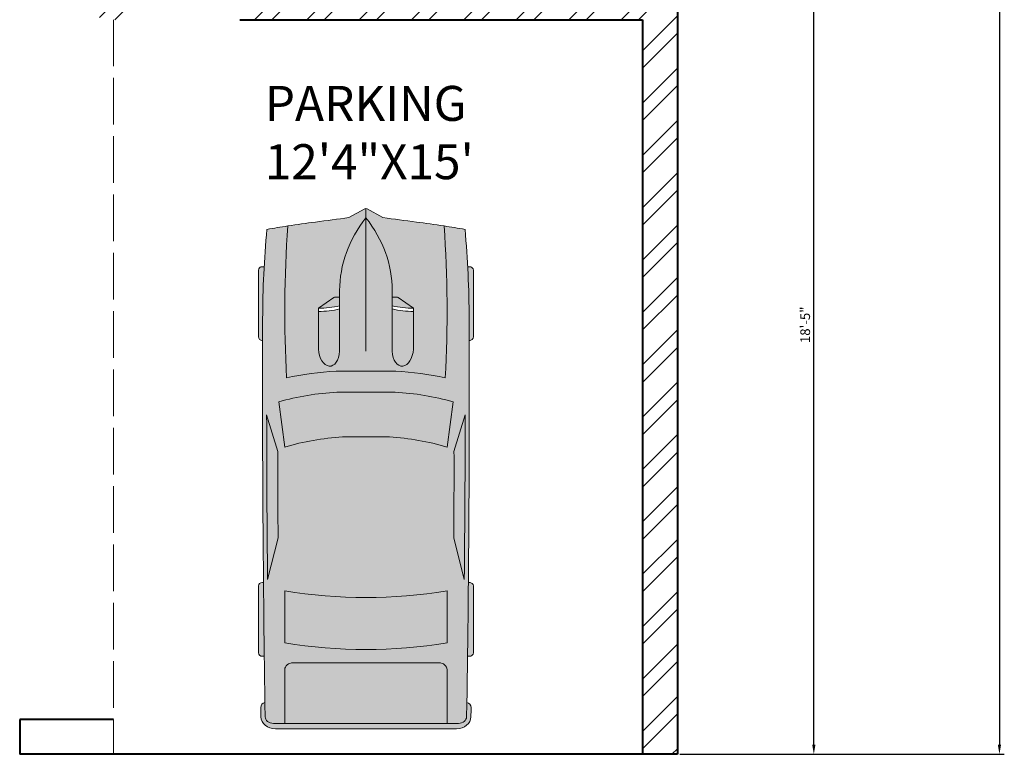
# Model space of a CAD drawing. Units: inches. Extents: x 1143 to 1626, y 7431 to 8140.
# Tile 2 of 4: x 1373 to 1626, y 7467 to 7656. Entities that reach past the tile are written whole.
import ezdxf

# ---------------------------------------------------------------- set-up
doc = ezdxf.new("R2010")
doc.units = ezdxf.units.IN
doc.linetypes.add('ACAD_ISO02W100', pattern=[15, 12, -3])
for name, color, linetype, lineweight in [('A-ANNO-DIMS', 4, 'Continuous', 18), ('A-EQPM-PATT', 9, 'Continuous', 13), ('A-EQPM-VEHC', 8, 'Continuous', 18), ('A-FLOR-PRKG', 2, 'ACAD_ISO02W100', 18), ('A-WALL', 2, 'Continuous', 40), ('A-WALL-PATT', 7, 'Continuous', 13)]:
    doc.layers.add(name, color=color, linetype=linetype, lineweight=lineweight)
doc.layers.add('A-AREA-IDEN', color=40, linetype='Continuous', lineweight=25, true_color=0xf8d731)
doc.styles.get("Standard").update_dxf_attribs({"font": 'arial.ttf'})
doc.dimstyles.new('ISO-25', dxfattribs={"dimtxt": 2.5, "dimasz": 2.5, "dimexe": 1.25, "dimexo": 0.625, "dimtad": 1, "dimdec": 0, "dimlunit": 3, "dimtxsty": 'Standard', "dimcen": 2.5, "dimadec": 0, "dimazin": 0, "dimtfac": 1, "dimtdec": 0, "dimtmove": 0, "dimatfit": 3, "dimfxl": 1, "dimarcsym": 0})

# ---------------------------------------------------------------- blocks, each defined once
blk = doc.blocks.new('*U56')
for p, q in [((536.0433148737552, 950.1792138851854), (536.0433148737552, 935.5404748014407)), ((1182.463644577746, 987.7673041878503), (567.7039087844591, 987.7673041878503)), ((1214.124238488447, 949.7089586534819), (1214.124238488447, 950.1792138851854)), ((2234.827175480885, 809.5287016048088), (1898.878785383111, 912.4126225124705)), ((3440.463608272525, 941.6679440245914), (3440.463608272525, 950.1792138851854)), ((3472.124202183229, 987.7673041878503), (4086.88393797651, 987.767304187848)), ((4118.544531887212, 950.1792138851804), (4118.544531887212, 934.0601128753084)), ((3411.559256322833, 904.3494681924599), (3029.921878250559, 807.1504809911063)), ((4736.411271353851, -850.8646766016326), (4736.411271353883, 850.864676601626)), ((4785.334832293326, -832.0706314503777), (4785.334832293357, 832.0706314502926)), ((1778.76917512805, 801.0177247054045), (2194.716249451875, 745.5217224176465)), ((3515.941238262737, 745.5217224176508), (3994.062813016633, 745.5217224176508)), ((4736.411271353883, 745.5217224176529), (4242.012185201922, 745.5217224176529)), ((4178.690997380514, 670.345541812321), (4178.690997380509, -670.3455418123318)), ((819.5542361210883, 295.2827619512633), (917.6699264680983, 436.1082195367583)), ((917.6699264680983, 436.1082195367583), (1293.848362214069, 436.1082195367583)), ((815.9220749762081, 241.4481679439487), (815.9220749762081, 283.3039660446585)), ((1496.485716216861, -273.6820371142997), (1496.485716216861, 273.6820371142868)), ((756.2288711996046, 241.4481679439487), (1312.764151599097, 241.4481679439487)), ((1690.372337881975, -267.4332505757059), (1690.372337881975, 267.4332505756928)), ((2101.521373270556, 215.7994139342878), (2101.521373270556, -215.7994139342835)), ((4736.411271353883, -267.4332505757059), (4736.411271353883, 267.4332505756928)), ((82.96813941916749, 155.6585683733955), (2.596917328392246, 10.3141998552517)), ((-1.1252e-12, -6.4972e-12), (1312.764151599097, -6.4972e-12)), ((2.596917328392246, -10.31419985525964), (82.96813941916749, -155.6585683734063)), ((756.2288711996046, -241.4481679439617), (1312.764151599097, -241.4481679439617)), ((815.9220749762081, -241.4481679439617), (815.9220749762081, -283.3039660446715)), ((819.5542361210883, -295.2827619512763), (917.6699264680983, -436.1082195367712)), ((917.6699264680983, -436.1082195367712), (1293.848362214069, -436.1082195367712)), ((2194.716249451869, -745.5217224176688), (1778.769175128041, -801.0177247054262)), ((2234.827175480882, -809.5287016048153), (1898.878785383109, -912.4126225124726)), ((3411.559256322828, -904.349468192473), (3029.921878250557, -807.150480991115)), ((3994.062813016633, -745.5217224176616), (3515.941238262737, -745.5217224176638)), ((4242.012185201917, -745.5217224176638), (4736.411271353857, -745.5217224176594)), ((536.0433148737552, -950.1792138851984), (536.0433148737552, -935.5404748014537)), ((1182.463644577746, -987.7673041878633), (567.7039087844591, -987.7673041878633)), ((1214.124238488447, -949.7089586534948), (1214.124238488447, -950.1792138851984)), ((3440.463608272523, -941.6679440246044), (3440.463608272523, -950.1792138851984)), ((3472.124202183229, -987.7673041878633), (4086.883937976504, -987.767304187861)), ((4118.544531887212, -950.1792138851933), (4118.544531887212, -934.0601128753214))]:
    blk.add_line(p, q)
for centre, major_axis, ratio, start_param, end_param in [((6757.162543998887, -699.1204428451242), (4.9938223e-09, 7958.017136535005), 0.8423038695435286, 1.367075990158062, 1.391760499156098), ((1046.255263051279, -12467.92283887244), (3.2861e-12, 13417.14359589015), 0.8423038695439741, 0.0028100083536837, 0.0755983031096952), ((567.7039087844591, 950.1792138851861), (5.296e-13, -37.5880903026662), 0.842303869543976, 3.141592653589776, 4.712388980384677), ((1637.842620806017, -268112.68896731), (4.8454159e-09, 269062.8681811952), 0.842303869543847, -0.0133969486112073, 0.0027970409639888), ((1182.463644577746, 950.1792138851861), (5.601e-13, 37.58809030266621), 0.8423038695439758, -1.570796326794884, 1.73e-14), ((1637.842620802809, -268112.6889680619), (4.87113144e-08, -269025.2800916445), 0.8423038695482963, 3.133765086725325, 3.140440689641252), ((3472.124202183229, 950.1792138851861), (5.988e-12, -37.5880903026662), 0.8423038695439762, 3.141592653589603, 4.712388980384554), ((4086.88393797651, 950.179213885181), (1.4197e-12, 37.5880903026662), 0.842303869543976, -1.570796326794865, 4.44e-14), ((4587.952203166941, 910.2894362332722), (1.8792e-12, 56.38213545399769), 0.8423038695439691, -0.0130174256259048, 1.249894140392862), ((1637.84262086767, -268131.4830124673), (3.42859201765e-05, 269120.9512111412), 0.8423038681351471, -0.0133969484821159, -0.0130174254969711), ((4673.090083532475, 850.8646766015395), (7.5e-15, -75.17618060533067), 0.8423038695439952, 1.570796326796048, 3.128195704978389), ((4673.090083532448, 832.070631450172), (2.1733e-12, -133.2592106239272), 0.8423038695439737, 1.570796326795794, 3.128195704978164), ((951.8333444315502, -15086.63944974413), (1.5767e-12, -15832.53653317094), 0.8423038695439826, 3.09604606856106, 3.200911180495224), ((3413.769624379244, 136.8410185571329), (1.08602e-11, -2280.347340451234), 0.84230386954398, 4.44948196380473, 4.652344057257214), ((3436.395912346701, 136.8410185571553), (5.76965e-11, 2077.023647078763), 0.8423038695439563, 1.245306111696802, 1.507880129813836), ((3799.722190048092, 71.1058404433382), (2.17448e-11, -2021.323467232052), 0.842303869543983, 4.372215489277867, 4.640744122441986), ((2433.035484508693, -93125.37499596032), (4.952654e-09, -93935.19844392464), 0.8423038695446962, 3.134048706297306, 3.14409775411291), ((433.884764992104, -3.6096e-12), (1.7438e-12, 3734.255266801694), 0.8423038695439766, 4.511394369635731, 4.913383591133647), ((912.0063397460013, -3.6096e-12), (1.7438e-12, 3734.255266801694), 0.8423038695439766, 4.511394369635731, 4.913383591133647), ((4242.012185201922, 670.3455418123216), (3.5405e-12, 75.17618060533239), 0.842303869543976, 5.55e-14, 1.57079632679492), ((6583.045501169266, -699.1204428451198), (3.826807e-09, -7754.693443154298), 0.8423038695443791, 4.528606069860317, 4.561837674556238), ((-5194.164488957196, 1330.879982200552), (1.0466145e-09, -6374.389491984369), 0.8423038695441164, 1.385369446298923, 1.434372047871027), ((331.12799165183, 432.0470009052715), (3.125e-11, 696.3661584994836), 0.8423038695439277, 4.435146050259648, 4.718221029521873), ((360.7019022476185, 432.0470009052715), (3.125e-11, 696.3661584994836), 0.8423038695439277, 4.435146050259648, 4.718221029521873), ((1290.073045555822, 338.7781937403542), (161.0379696969085, -9.057857958340485), 0.6038335755719145, -1.39555193967809, 1.581314658479915), ((831.7523719315589, 283.3039660446593), (3.3347e-12, 18.79404515133458), 0.8423038695439091, 0.8797135699495516, 1.570796326795045), ((756.2288711996046, -1185.240851913765), (1.2998e-12, 1426.689019857713), 0.842303869543976, 7e-16, 0.5903187773915901), ((15.83029695535095, -3.6096e-12), (1.9e-15, -18.79404515133476), 0.842303869543842, 4.131459131953847, 5.293318828815531), ((756.2288711996046, 1185.240851913753), (1.01699e-11, 1426.689019857713), 0.8423038695439736, 2.55127387619821, 3.141592653589801), ((-5194.164488957196, -1330.879982200562), (1.0234792e-09, 6374.389491984348), 0.8423038695441192, -1.43437204787103, -1.385369446298926), ((331.12799165183, -432.0470009052816), (3.1922e-11, -696.3661584994801), 0.842303869543932, 1.564964277657711, 1.848039256919935), ((360.7019022476185, -432.0470009052816), (3.1922e-11, -696.3661584994801), 0.842303869543932, 1.564964277657711, 1.848039256919935), ((3436.395912346742, -136.8410185572101), (8.13766e-11, -2077.023647078826), 0.8423038695439492, -1.50788012981387, -1.245306111696839), ((3799.722190048497, -71.10584044329416), (1.038796e-10, -2021.323467232635), 0.8423038695439419, -1.499151468852248, -1.230622835688196), ((831.7523719315589, -283.3039660446737), (3.3028e-12, -18.79404515133458), 0.8423038695439093, 4.712388980384541, 5.403471737230034), ((3413.769624379237, -136.841018557156), (1.090899e-10, -2280.347340451348), 0.8423038695439354, -1.510751403667474, -1.307889310215002), ((6583.045501169163, 699.1204428449458), (2.756795e-10, 7754.693443157768), 0.8423038695439974, 1.721347632622872, 1.754579237318777), ((6757.162543998887, 699.1204428451076), (2.2231118e-09, 7958.017136528592), 0.8423038695441819, 1.749832154434603, 1.774516663432659), ((951.8333444315729, 15086.63944974408), (2.97009e-11, -15832.5365331709), 0.8423038695439528, -0.0593185269054384, 0.0455465850287298), ((4242.012185201917, -670.3455418123318), (2.579e-13, -75.17618060533128), 0.8423038695439885, 4.712388980384686, 6.283185307179581), ((2433.03548450906, 93125.37499596029), (4.1600574e-09, -93935.19844392457), 0.8423038695447548, -0.0025051005232382, 0.007543947292366), ((1637.842620803916, 268112.6889680615), (4.0766478e-08, -269025.280091644), 0.8423038695397146, 0.0011519639481523, 0.0078275668641468), ((4673.090083532448, -850.8646766015358), (2.354e-13, 75.17618060532999), 0.8423038695439732, 3.154989602201626, 4.71238898038339), ((4673.090083532349, -832.0706314501077), (6.1679e-12, -133.2592106240062), 0.8423038695439807, 0.0133969486110846, 1.570796326792831), ((1046.255263051284, 12467.92283887242), (3.49903e-10, -13417.14359589015), 0.8423038695440652, -0.0755983031097181, -0.0028100083537155), ((567.7039087844591, -950.1792138851977), (5.601e-13, 37.58809030266621), 0.8423038695439758, 1.570796326794908, 3.14159265358981), ((1637.842620801787, 268112.6889680619), (1.55395844e-08, 269062.868181947), 0.8423038695458147, 3.138795612625926, 3.154989602201039), ((1182.463644577746, -950.1792138851977), (5.296e-13, -37.5880903026662), 0.842303869543976, -1.69e-14, 1.570796326794884), ((3472.124202183229, -950.1792138851955), (3.96e-13, -37.58809030266733), 0.8423038695440105, -1.570796326794875, -1.27e-14), ((4086.883937976504, -950.1792138851933), (5.0003e-12, 37.58809030266732), 0.8423038695440109, 3.141592653589951, 4.712388980384771), ((4587.952203166856, -910.2894362333229), (5.777e-12, -56.38213545402103), 0.8423038695439803, -1.249894138785958, 0.0130174256254374), ((1637.842620726191, 268131.4830135791), (2.37878358395e-05, 269120.9512123862), 0.8423038705260315, 3.154610079306566, 3.154989602290631)]:
    blk.add_ellipse(centre, major_axis=major_axis, ratio=ratio, start_param=start_param, end_param=end_param)
at = {"extrusion": (0, 0, -1)}
blk.add_ellipse((1290.073045555822, -338.7781937403665), major_axis=(161.0379696969085, 9.057857958340424), ratio=0.6038335755719145, start_param=-1.39555193967809, end_param=1.581314658479915, dxfattribs=at)
blk = doc.blocks.new('*D59')
at = {"layer": 'A-ANNO-DIMS', "color": 0, "lineweight": -2, "transparency": 16777216}
for p, q in [((1542.475441917873, 8067.395884901202), (1625.931990479295, 8067.395884901202)), ((1624.681990479295, 8064.895884901202), (1624.681990479295, 7469.895884901203)), ((1542.475441917873, 7467.395884901204), (1625.931990479295, 7467.395884901204))]:
    blk.add_line(p, q, dxfattribs=at)
at = {"layer": 'A-ANNO-DIMS', "color": 0, "transparency": 16777216}
for points in [[(1624.265323812629, 8064.895884901202), (1625.098657145962, 8064.895884901202), (1624.681990479295, 8067.395884901202)], [(1624.265323812629, 7469.895884901203), (1625.098657145963, 7469.895884901203), (1624.681990479295, 7467.395884901204)]]:
    blk.add_solid(points, dxfattribs=at)
at = {"layer": 'Defpoints', "color": 0, "transparency": 16777216}
for p in [(1541.850441917873, 8067.395884901202), (1541.850441917873, 7467.395884901204), (1624.681990479295, 7467.395884901204)]:
    blk.add_point(p, dxfattribs=at)
at = {"layer": 'A-ANNO-DIMS', "color": 0, "transparency": 16777216, "insert": (1615.88782267575, 7767.395884901201), "char_height": 2.5, "attachment_point": 5, "rotation": 90}
blk.add_mtext("{\\H6.4x;50'}", dxfattribs=at)
blk = doc.blocks.new('*D94')
at = {"layer": 'A-ANNO-DIMS', "color": 0, "lineweight": -2, "transparency": 16777216}
for p, q in [((1542.475442000001, 7688.395885000004), (1578.200442000001, 7688.395885000004)), ((1576.950442000002, 7469.895885000004), (1576.950442000002, 7685.895885000004)), ((1542.475442000001, 7467.395885000003), (1578.200442000002, 7467.395885000003))]:
    blk.add_line(p, q, dxfattribs=at)
at = {"layer": 'A-ANNO-DIMS', "color": 0, "transparency": 16777216}
for points in [[(1576.533775333335, 7685.895885000004), (1577.367108666668, 7685.895885000004), (1576.950442000002, 7688.395885000004)], [(1576.533775333335, 7469.895885000004), (1577.367108666669, 7469.895885000004), (1576.950442000002, 7467.395885000003)]]:
    blk.add_solid(points, dxfattribs=at)
at = {"layer": 'Defpoints', "color": 0, "transparency": 16777216}
for p in [(1541.850442000001, 7688.395885000004), (1576.950442000002, 7688.395885000004), (1541.850442000001, 7467.395885000003)]:
    blk.add_point(p, dxfattribs=at)
at = {"layer": 'A-ANNO-DIMS', "color": 0, "transparency": 16777216, "insert": (1575.049009530699, 7577.895885000002), "char_height": 2.5, "attachment_point": 5, "rotation": 90}
blk.add_mtext('18\'-5"', dxfattribs=at)

msp = doc.modelspace()

# ---------------------------------------------------------------- hatches: boundary and pattern name
at = {"layer": 'A-EQPM-PATT'}
h = msp.add_hatch(color=256, dxfattribs=at)
h.dxf.hatch_style = 1
edge = h.paths.add_edge_path()
edge.add_ellipse((1039.678384205543, 7581.215646983221), major_axis=(442.95140415634, 3.6663e-12), ratio=0.8423038695438162, start_angle=-2.198540565955638, end_angle=2.863714607837108)
edge.add_ellipse((1442.202119620892, 7423.669613427368), major_axis=(216.9552770171625, 6.603309e-10), ratio=0.8423038695464521, start_angle=77.55537270638033, end_angle=79.79046100268101)
edge.add_ellipse((1498.996022280016, 7753.163986690991), major_axis=(178.3381184811209, 2.862326e-10), ratio=0.842303869545449, start_angle=257.4450673557707, end_angle=260.7434339927064, ccw=False)
edge.add_line((1466.116516563501, 7605.524137399554), (1462.050175583554, 7607.772706073581))
edge.add_ellipse((1461.761612263391, 7607.402472025788), major_axis=(-0.5258063780318869, 7.886e-13), ratio=0.8423038695429472, start_angle=232.0668695402551, end_angle=270.0000000000859)
edge.add_line((1461.761612263391, 7607.845360772635), (1461.761612263391, 7605.40214945713))
edge.add_ellipse((1428.601789861041, 7586.688129291778), major_axis=(-39.91488687339462, 4.1769e-12), ratio=0.8423038695440169, start_angle=180.000000000006, end_angle=209.4385695979854, ccw=False)
edge.add_line((1468.516676734435, 7586.688129291778), (1468.516676734435, 7585.01807545195))
edge.add_line((1468.516676734435, 7585.01807545195), (1469.811288061556, 7585.01807545195))
edge.add_ellipse((1469.687688372524, 7584.575186705103), major_axis=(0.5258063780289138, 6.2901e-12), ratio=0.8423038695477099, start_angle=45.519789116729726, end_angle=89.99999999931458, ccw=False)
edge.add_line((1470.022822572645, 7584.916457440465), (1473.962736688602, 7582.171446701479))
edge.add_line((1473.962736688602, 7582.171446701479), (1473.962736688602, 7571.646994982835))
edge.add_ellipse((1471.239706711519, 7571.752618097072), major_axis=(0.2534142834889348, 4.505405349943914), ratio=0.6038335755718542, start_angle=106.3425919543661, end_angle=270.9979857250239, ccw=False)
edge.add_line((1468.516676734435, 7571.117782531546), (1468.516676734435, 7586.688129291778))
edge.add_ellipse((1428.601789861041, 7586.688129291778), major_axis=(-39.91488687339462, 4.1769e-12), ratio=0.8423038695440169, start_angle=180.000000000006, end_angle=209.4385695979854)
edge.add_ellipse((1494.92143466574, 7586.688129291778), major_axis=(-39.9148868733946, 1.8282e-12), ratio=0.8423038695439518, start_angle=-29.43856959797676, end_angle=2.6254e-12)
edge.add_line((1455.006547792345, 7586.688129291778), (1455.006547792345, 7571.117782531546))
edge.add_ellipse((1452.283517815262, 7571.752618097072), major_axis=(-0.2534142834889348, 4.505405349943914), ratio=0.6038335755718542, start_angle=89.0020142749762, end_angle=253.6574080456339, ccw=False)
edge.add_line((1449.560487838178, 7571.646994982835), (1449.560487838178, 7582.171446701479))
edge.add_line((1449.560487838178, 7582.171446701479), (1453.595642479137, 7584.982813268593))
edge.add_ellipse((1453.835536154257, 7584.575186705103), major_axis=(-0.525806378028914, 6.2893e-12), ratio=0.8423038695477096, start_angle=-89.99999999931458, end_angle=-45.519789116729726, ccw=False)
edge.add_line((1453.835536154257, 7585.01807545195), (1455.006547792345, 7585.01807545195))
edge.add_line((1455.006547792345, 7585.01807545195), (1455.006547792345, 7586.688129291778))
edge.add_ellipse((1494.92143466574, 7586.688129291778), major_axis=(-39.9148868733946, 1.8282e-12), ratio=0.8423038695439518, start_angle=-29.438569597976823, end_angle=2.6716406864579767e-12, ccw=False)
edge.add_line((1461.761612263391, 7605.40214945713), (1461.761612263391, 7607.845360772635))
edge.add_ellipse((1461.761612263391, 7607.402472025788), major_axis=(-0.5258063780318869, 7.886e-13), ratio=0.8423038695429472, start_angle=270.0000000000859, end_angle=307.9331304599605)
edge.add_line((1461.473048943226, 7607.772706073581), (1457.406707963279, 7605.524137399554))
edge.add_ellipse((1424.527202246764, 7753.163986690991), major_axis=(-178.3381184811248, 2.85599e-10), ratio=0.8423038695454304, start_angle=99.25656600729332, end_angle=102.5549326442291, ccw=False)
edge.add_ellipse((1481.321104905884, 7423.669613427371), major_axis=(-216.9552770172325, 5.765085e-10), ratio=0.8423038695461753, start_angle=-79.79046100270455, end_angle=-77.55537270640374)
edge.add_ellipse((1883.844840321237, 7581.215646983221), major_axis=(-442.9514041563389, 7.3054e-12), ratio=0.8423038695438002, start_angle=-2.863714607836754, end_angle=2.198540565956014)
edge.add_ellipse((1457.933171938046, 7512.337351337953), major_axis=(-63.79792993373228, 4.06461e-11), ratio=0.8423038695444189, start_angle=-85.9175893088132, end_angle=-72.2800467772135, ccw=False)
edge.add_line((1454.104731612702, 7565.977751756898), (1469.418492914078, 7565.977751756898))
edge.add_ellipse((1465.590052588734, 7512.337351337953), major_axis=(63.79792993373165, 4.44426e-11), ratio=0.8423038695444265, start_angle=72.2800467772093, end_angle=85.91758930880928, ccw=False)
edge = h.paths.add_edge_path()
edge.add_ellipse((1480.516061267415, 7489.165372259944), major_axis=(-2.103225512126755, 1.679e-12), ratio=0.842303869543697, start_angle=180.0000000000457, end_angle=270.0000000000457)
edge.add_line((1480.516061267415, 7490.936927247331), (1443.007163259365, 7490.936927247331))
edge.add_ellipse((1443.007163259365, 7489.165372259944), major_axis=(2.103225512126754, 1.6786e-12), ratio=0.842303869543697, start_angle=89.99999999995427, end_angle=179.9999999999543)
edge.add_line((1440.903937747239, 7489.165372259944), (1440.903937747239, 7475.333427582867))
edge.add_line((1440.903937747239, 7475.333427582867), (1482.619286779542, 7475.333427582866))
edge.add_line((1482.619286779542, 7475.333427582866), (1482.619286779542, 7489.165372259944))
h = msp.add_hatch(color=256, dxfattribs=at)
h.dxf.hatch_style = 1
edge = h.paths.add_edge_path()
edge.add_ellipse((-6039.303791968246, 7562.022969196078), major_axis=(7527.648839937518, 6.974655e-10), ratio=0.8423038695462727, start_angle=-0.3838667787978237, end_angle=0.0902290885890152)
edge.add_ellipse((-6039.303791968246, 7562.022969196078), major_axis=(7527.648839937518, 6.974655e-10), ratio=0.8423038695462727, start_angle=0.0902290885890152, end_angle=0.134986576852948)
edge.add_ellipse((1112.942968022728, 7578.573977952608), major_axis=(-375.3752649245584, 1.99436e-11), ratio=0.8423038695442169, start_angle=180.1356123904414, end_angle=182.1799503136482)
edge.add_ellipse((1112.942968022728, 7578.573977952608), major_axis=(-375.3752649245584, 1.99436e-11), ratio=0.8423038695442169, start_angle=182.1799503136482, end_angle=183.650427585702)
edge.add_ellipse((1442.202119620892, 7418.798291106567), major_axis=(222.6437221564754, 1.774424e-10), ratio=0.8423038695446471, start_angle=76.2194710104564, end_angle=77.87403444767025)
edge.add_ellipse((1039.678384205543, 7581.215646983221), major_axis=(442.95140415634, 3.6663e-12), ratio=0.8423038695438162, start_angle=-2.198540565955625, end_angle=2.863714607837096, ccw=False)
edge.add_ellipse((1465.590052588734, 7512.337351337953), major_axis=(63.79792993373165, 4.44426e-11), ratio=0.8423038695444265, start_angle=72.28004677720928, end_angle=85.91758930880933)
edge.add_line((1469.418492914078, 7565.977751756898), (1454.104731612702, 7565.977751756898))
edge.add_ellipse((1457.933171938046, 7512.337351337953), major_axis=(-63.79792993373228, 4.06461e-11), ratio=0.8423038695444189, start_angle=-85.91758930881322, end_angle=-72.28004677721358)
edge.add_ellipse((1883.844840321237, 7581.215646983221), major_axis=(-442.9514041563389, 7.3054e-12), ratio=0.8423038695438002, start_angle=-2.863714607836698, end_angle=2.198540565956023, ccw=False)
edge.add_ellipse((1481.321104905889, 7418.798291106567), major_axis=(-222.6437221561361, 5.461424e-10), ratio=0.842303869545886, start_angle=-77.87403444757535, end_angle=-76.21947101036163)
edge.add_ellipse((1810.580256504053, 7578.573977952607), major_axis=(375.3752649245585, 6.42025e-11), ratio=0.8423038695444667, start_angle=176.3495724142911, end_angle=177.8200496863449)
edge.add_ellipse((1810.580256504053, 7578.573977952607), major_axis=(375.3752649245585, 6.42025e-11), ratio=0.8423038695444667, start_angle=177.8200496863449, end_angle=179.8643876095517)
edge.add_ellipse((8962.827016516063, 7562.022969196194), major_axis=(-7527.648839958555, 1.993663e-10), ratio=0.8423038695442729, start_angle=-0.1349865768554994, end_angle=-0.090229088591682)
edge.add_ellipse((8962.827016516063, 7562.022969196194), major_axis=(-7527.648839958555, 1.993663e-10), ratio=0.8423038695442729, start_angle=-0.090229088591682, end_angle=0.383866778793832)
edge.add_ellipse((8962.827016516063, 7562.022969196194), major_axis=(-7527.648839958555, 1.993663e-10), ratio=0.8423038695442729, start_angle=0.383866778793832, end_angle=0.5282714718188681)
edge.add_ellipse((8962.827016516063, 7562.022969196194), major_axis=(-7527.648839958555, 1.993663e-10), ratio=0.8423038695442729, start_angle=0.5282714718188681, end_angle=0.6465540970624511)
edge.add_ellipse((1437.956727780222, 7477.104982570255), major_axis=(2.10322551212646, 1.4268e-12), ratio=0.8423038695438149, start_angle=180.6465540970471, end_angle=269.9999999998729)
edge.add_line((1437.956727780219, 7475.333427582867), (1440.903937747239, 7475.333427582867))
edge.add_line((1440.903937747239, 7475.333427582867), (1440.903937747239, 7489.398770874538))
edge.add_ellipse((1443.007163259365, 7489.165372259944), major_axis=(2.103225512126754, 1.6786e-12), ratio=0.842303869543697, start_angle=89.9999999999543, end_angle=179.9999999999543, ccw=False)
edge.add_line((1443.007163259365, 7490.936927247331), (1480.793156770639, 7490.936927247331))
edge.add_ellipse((1480.516061267415, 7489.165372259944), major_axis=(-2.103225512126755, 1.679e-12), ratio=0.842303869543697, start_angle=180.0000000000458, end_angle=270.0000000000457, ccw=False)
edge.add_line((1482.619286779542, 7489.165372259944), (1482.619286779542, 7475.333427582866))
edge.add_line((1482.619286779542, 7475.333427582866), (1485.566496746561, 7475.333427582866))
edge.add_ellipse((1485.566496746559, 7477.104982570255), major_axis=(2.103225512126458, 1.1705e-12), ratio=0.842303869543816, start_angle=-89.99999999995839, end_angle=-0.6465540970932105)
edge.add_ellipse((-6039.303791968246, 7562.022969196078), major_axis=(7527.648839937518, 6.974655e-10), ratio=0.8423038695462727, start_angle=-0.6465540970672118, end_angle=-0.6186431963245203)
edge.add_ellipse((-6039.303791968246, 7562.022969196078), major_axis=(7527.648839937518, 6.974655e-10), ratio=0.8423038695462727, start_angle=-0.6186431963245203, end_angle=-0.5282714718232633)
edge.add_ellipse((-6039.303791968246, 7562.022969196078), major_axis=(7527.648839937518, 6.974655e-10), ratio=0.8423038695462727, start_angle=-0.5282714718232633, end_angle=-0.3838667787978237)
edge = h.paths.add_edge_path(flags=16)
edge.add_line((1439.179732337113, 7523.076369547308), (1436.460368464291, 7512.399191437433))
edge.add_ellipse((8962.827016516048, 7562.022969196134), major_axis=(7526.597227202479, 2.1947994e-09), ratio=0.8423038695377735, start_angle=180.0555943134824, end_angle=180.3777641938929, ccw=False)
edge.add_line((1436.234783289076, 7554.719885739243), (1439.113196178613, 7545.320961517211))
edge.add_ellipse((4067.156870984121, 7539.775630949648), major_axis=(-2628.051921008733, 2.52533e-11), ratio=0.8423038695471943, start_angle=-0.1208973690324235, end_angle=0.3640763488906122)
edge = h.paths.add_edge_path(flags=16)
edge.add_ellipse((1459.772263822471, 7501.539445990141), major_axis=(56.55114492797071, 8.197e-13), ratio=0.8423038695440553, start_angle=94.87006959713516, end_angle=112.7919148775863)
edge.add_line((1440.903937747239, 7546.443156370158), (1439.351310214252, 7558.080226667799))
edge.add_ellipse((1457.933171938045, 7511.704329206278), major_axis=(-58.10948479492556, 2.9454e-12), ratio=0.8423038695440394, start_angle=-85.7225790369431, end_angle=-68.16504620328902, ccw=False)
edge.add_line((1454.279555701423, 7560.553330273092), (1469.243668825358, 7560.553330273092))
edge.add_ellipse((1465.590052588735, 7511.704329206279), major_axis=(58.10948479492538, 4.597e-12), ratio=0.842303869544011, start_angle=68.16504620328561, end_angle=85.7225790369398, ccw=False)
edge.add_line((1484.171914312528, 7558.080226667799), (1482.619286779541, 7546.443156370158))
edge.add_ellipse((1463.750960704312, 7501.539445990153), major_axis=(56.55114492795597, 1.7238e-12), ratio=0.8423038695440801, start_angle=67.20808512240856, end_angle=85.12993040286277)
edge.add_line((1467.799094205594, 7549.050496083426), (1455.724130321186, 7549.050496083426))
edge = h.paths.add_edge_path(flags=16)
edge.add_ellipse((1461.761612263391, 7595.706442571333), major_axis=(-104.4743279412191, 7.6e-14), ratio=0.8423038695440698, start_angle=76.4018653097694, end_angle=103.5981346902307)
edge.add_line((1482.619286779542, 7509.478866865816), (1482.619286779542, 7496.102322781993))
edge.add_ellipse((1461.761612263391, 7582.329898487511), major_axis=(-104.4743279412456, 6.4e-15), ratio=0.8423038695438568, start_angle=76.40186530976962, end_angle=103.5981346902305, ccw=False)
edge.add_line((1440.903937747239, 7496.102322781993), (1440.903937747239, 7509.478866865816))
edge = h.paths.add_edge_path(flags=16)
edge.add_ellipse((-1143.633646457342, 7539.775630949661), major_axis=(2628.051921008736, 4.290663e-10), ratio=0.8423038695493088, start_angle=-0.3640763488997026, end_angle=0.1208973690233077)
edge.add_line((1484.41002834817, 7545.320961517219), (1487.288441237708, 7554.719885739253))
edge.add_ellipse((-6039.303791989281, 7562.022969196168), major_axis=(7526.597227202493, 5.536414e-10), ratio=0.8423038695434923, start_angle=-0.37776419391400395, end_angle=-0.05559431350360455, ccw=False)
edge.add_line((1487.062856062488, 7512.399191437438), (1484.343492189669, 7523.076369547303))
h = msp.add_hatch(color=256, dxfattribs=at)
h.dxf.hatch_style = 1
edge = h.paths.add_edge_path()
edge.add_ellipse((1810.580256504053, 7578.573977952607), major_axis=(375.3752649245585, 6.42025e-11), ratio=0.8423038695444667, start_angle=177.820049686345, end_angle=179.8643876095518, ccw=False)
edge.add_line((1435.587728748884, 7592.848323594513), (1435.178176557506, 7592.848323594513))
edge.add_ellipse((1435.178176557506, 7591.962546100818), major_axis=(-1.051612756063605, 1.3637e-12), ratio=0.8423038695439471, start_angle=-89.9999999999257, end_angle=7.42938e-11)
edge.add_line((1434.126563801443, 7591.962546100818), (1434.126563801443, 7574.763237094463))
edge.add_ellipse((1435.178176557506, 7574.763237094463), major_axis=(-1.051612756063605, 3.0636e-12), ratio=0.8423038695439471, start_angle=1.66912e-10, end_angle=90.0000000001669)
edge.add_line((1435.178176557494, 7573.87745960077), (1435.191333022661, 7573.87745960077))
edge.add_ellipse((8962.827016516063, 7562.022969196194), major_axis=(-7527.648839958555, 1.993663e-10), ratio=0.8423038695442729, start_angle=-0.13498657685551052, end_angle=-0.0902290885916841, ccw=False)
edge = h.paths.add_edge_path()
edge.add_ellipse((1488.345047969274, 7591.962546100818), major_axis=(1.051612756063605, 3.2278e-12), ratio=0.8423038695439471, start_angle=-1.758599e-10, end_angle=89.99999999982413)
edge.add_line((1488.345047969274, 7592.848323594513), (1487.935495777897, 7592.848323594513))
edge.add_ellipse((1112.942968022728, 7578.573977952608), major_axis=(-375.3752649245584, 1.99436e-11), ratio=0.8423038695442169, start_angle=180.1356123904414, end_angle=182.1799503136482, ccw=False)
edge.add_ellipse((-6039.303791968246, 7562.022969196078), major_axis=(7527.648839937518, 6.974655e-10), ratio=0.8423038695462727, start_angle=0.09022908858912615, end_angle=0.1349865768530094, ccw=False)
edge.add_line((1488.331891504119, 7573.87745960077), (1488.345047969287, 7573.87745960077))
edge.add_ellipse((1488.345047969274, 7574.763237094463), major_axis=(1.051612756063605, 1.1996e-12), ratio=0.8423038695439471, start_angle=269.9999999999346, end_angle=359.9999999999346)
edge.add_line((1489.396660725338, 7574.763237094463), (1489.396660725338, 7591.962546100818))
h = msp.add_hatch(color=256, dxfattribs=at)
h.dxf.hatch_style = 1
edge = h.paths.add_edge_path()
edge.add_ellipse((1473.849114813065, 7597.753900459394), major_axis=(-19.48243524140747, 2.29375e-11), ratio=0.8423038695428267, start_angle=71.3325045074642, end_angle=90.39670986004552, ccw=False)
edge.add_line((1468.516676734435, 7581.970411766802), (1468.516676734435, 7571.117782531546))
edge.add_ellipse((1471.239706711519, 7571.752618097072), major_axis=(0.2534142834889348, 4.505405349943914), ratio=0.6038335755718542, start_angle=106.3425919543661, end_angle=270.9979857250238)
edge.add_line((1473.962736688602, 7571.646994982835), (1473.962736688602, 7581.344048943869))
edge = h.paths.add_edge_path()
edge.add_ellipse((1449.674109713715, 7597.753900459394), major_axis=(-19.48243524138126, 9.0814e-12), ratio=0.8423038695439155, start_angle=89.60329014004873, end_angle=108.66749549263, ccw=False)
edge.add_line((1449.560487838178, 7581.34404894387), (1449.560487838178, 7571.646994982835))
edge.add_ellipse((1452.283517815262, 7571.752618097072), major_axis=(-0.2534142834889348, 4.505405349943914), ratio=0.6038335755718542, start_angle=89.0020142749761, end_angle=253.6574080456339)
edge.add_line((1455.006547792345, 7571.117782531546), (1455.006547792345, 7581.970411766802))
edge = h.paths.add_edge_path()
edge.add_line((1455.006547792345, 7585.01807545195), (1453.835536154257, 7585.01807545195))
edge.add_ellipse((1453.835536154257, 7584.575186705103), major_axis=(-0.525806378028914, 6.2893e-12), ratio=0.8423038695477096, start_angle=-89.99999999931468, end_angle=-45.51978911672977)
edge.add_line((1453.500401954136, 7584.916457440465), (1449.560487838178, 7582.171446701479))
edge.add_ellipse((1449.674109713715, 7598.581298217002), major_axis=(-19.48243524135515, 1.89749e-11), ratio=0.8423038695450452, start_angle=89.60329014007783, end_angle=108.66749549266)
edge.add_line((1455.006547792345, 7582.797809524411), (1455.006547792345, 7585.01807545195))
edge = h.paths.add_edge_path()
edge.add_ellipse((1469.687688372524, 7584.575186705103), major_axis=(0.5258063780289138, 6.2901e-12), ratio=0.8423038695477099, start_angle=45.51978911672967, end_angle=89.9999999993146)
edge.add_line((1469.687688372524, 7585.01807545195), (1468.516676734435, 7585.01807545195))
edge.add_line((1468.516676734435, 7585.01807545195), (1468.516676734435, 7582.797809524411))
edge.add_ellipse((1473.849114813065, 7598.581298217002), major_axis=(19.48243524135507, 1.90528e-11), ratio=0.8423038695450485, start_angle=251.3325045073396, end_angle=270.3967098599219)
edge.add_line((1473.962736688602, 7582.171446701479), (1470.022822572645, 7584.916457440465))
edge = h.paths.add_edge_path()
edge.add_ellipse((-6039.303791989281, 7562.022969196168), major_axis=(7526.597227202493, 5.536414e-10), ratio=0.8423038695434923, start_angle=-0.3777641939140973, end_angle=-0.0555943135036058)
edge.add_line((1487.288441237708, 7554.719885739253), (1484.41002834817, 7545.320961517219))
edge.add_ellipse((-1143.633646457342, 7539.775630949661), major_axis=(2628.051921008736, 4.290663e-10), ratio=0.8423038695493088, start_angle=-0.36407634889968676, end_angle=0.12089736902328241, ccw=False)
edge.add_line((1484.343492189669, 7523.076369547303), (1487.062856062488, 7512.399191437438))
h = msp.add_hatch(color=256, dxfattribs=at)
h.dxf.hatch_style = 1
edge = h.paths.add_edge_path()
edge.add_ellipse((1465.590052588735, 7511.704329206279), major_axis=(58.10948479492538, 4.597e-12), ratio=0.842303869544011, start_angle=68.16504620328563, end_angle=85.72257903693978)
edge.add_line((1469.243668825358, 7560.553330273092), (1454.279555701423, 7560.553330273092))
edge.add_ellipse((1457.933171938045, 7511.704329206278), major_axis=(-58.10948479492556, 2.9454e-12), ratio=0.8423038695440394, start_angle=-85.72257903694315, end_angle=-68.16504620328898)
edge.add_line((1439.351310214252, 7558.080226667799), (1440.903937747239, 7546.443156370158))
edge.add_ellipse((1459.772263822471, 7501.539445990141), major_axis=(56.55114492797071, 8.197e-13), ratio=0.8423038695440553, start_angle=94.87006959713523, end_angle=112.79191487758641, ccw=False)
edge.add_line((1455.724130321186, 7549.050496083426), (1467.799094205594, 7549.050496083426))
edge.add_ellipse((1463.750960704312, 7501.539445990153), major_axis=(56.55114492795597, 1.7238e-12), ratio=0.8423038695440801, start_angle=67.20808512240859, end_angle=85.12993040286278, ccw=False)
edge.add_line((1482.619286779541, 7546.443156370158), (1484.171914312528, 7558.080226667799))
edge = h.paths.add_edge_path()
edge.add_ellipse((1461.761612263391, 7595.706442571333), major_axis=(-104.4743279412191, 7.6e-14), ratio=0.8423038695440698, start_angle=76.40186530976939, end_angle=103.59813469023072, ccw=False)
edge.add_line((1440.903937747239, 7509.478866865816), (1440.903937747239, 7496.102322781993))
edge.add_ellipse((1461.761612263391, 7582.329898487511), major_axis=(-104.4743279412456, 6.4e-15), ratio=0.8423038695438568, start_angle=76.40186530976948, end_angle=103.5981346902305)
edge.add_line((1482.619286779542, 7496.102322781993), (1482.619286779542, 7509.478866865816))
h = msp.add_hatch(color=256, dxfattribs=at)
h.dxf.hatch_style = 1
edge = h.paths.add_edge_path()
edge.add_ellipse((4067.156870984121, 7539.775630949648), major_axis=(-2628.051921008733, 2.52533e-11), ratio=0.8423038695471943, start_angle=-0.12089736903237736, end_angle=0.3640763488907055, ccw=False)
edge.add_line((1439.113196178613, 7545.320961517211), (1436.234783289076, 7554.719885739243))
edge.add_ellipse((8962.827016516048, 7562.022969196134), major_axis=(7526.597227202479, 2.1947994e-09), ratio=0.8423038695377735, start_angle=180.0555943134823, end_angle=180.3777641938928)
edge.add_line((1436.460368464291, 7512.399191437433), (1439.179732337113, 7523.076369547308))
h = msp.add_hatch(color=256, dxfattribs=at)
h.dxf.hatch_style = 1
edge = h.paths.add_edge_path()
edge.add_ellipse((1485.040690368526, 7477.104982570255), major_axis=(3.728231060068574, 7.337e-13), ratio=0.8423038695438233, start_angle=-89.99999999994495, end_angle=-0.6465540970816102)
edge.add_ellipse((-6039.829598346445, 7562.022969194353), major_axis=(-7529.273845483747, 8.251344458e-07), ratio=0.8423038683212265, start_angle=179.3534459092302, end_angle=179.3717627900635)
edge.add_ellipse((1487.229040247746, 7479.486909406539), major_axis=(-1.577419134094872, 1.8873e-12), ratio=0.8423038695437339, start_angle=179.371762783849, end_angle=248.4647566010657)
edge.add_ellipse((-6039.303791968246, 7562.022969196078), major_axis=(7527.648839937518, 6.974655e-10), ratio=0.8423038695462727, start_angle=-0.6465540970672237, end_angle=-0.6186431963245127, ccw=False)
edge.add_ellipse((1485.566496746559, 7477.104982570255), major_axis=(2.103225512126458, 1.1705e-12), ratio=0.842303869543816, start_angle=-89.99999999995839, end_angle=-0.6465540970932011, ccw=False)
edge.add_line((1485.566496746561, 7475.333427582866), (1437.956727780219, 7475.333427582867))
edge.add_ellipse((1437.956727780222, 7477.104982570255), major_axis=(2.10322551212646, 1.4268e-12), ratio=0.8423038695438149, start_angle=180.6465540970472, end_angle=269.9999999998729, ccw=False)
edge.add_ellipse((8962.827016516063, 7562.022969196194), major_axis=(-7527.648839958555, 1.993663e-10), ratio=0.8423038695442729, start_angle=0.5282714718189254, end_angle=0.6465540970625057, ccw=False)
edge.add_ellipse((1436.294184279033, 7479.48690940654), major_axis=(1.577419134095759, 6.785e-13), ratio=0.8423038695440649, start_angle=111.5352435039945, end_angle=180.6282372161284)
edge.add_ellipse((8963.35282290433, 7562.022969198308), major_axis=(-7529.273845518149, 6.107500749e-07), ratio=0.8423038704380847, start_angle=0.62823722089072, end_angle=0.6465541017237717)
edge.add_ellipse((1438.482534158256, 7477.104982570257), major_axis=(3.728231060070373, 7.436e-13), ratio=0.842303869543905, start_angle=180.6465540970446, end_angle=269.9999999998558)
edge.add_line((1438.482534158249, 7473.964679121806), (1485.04069036853, 7473.964679121806))
edge = h.paths.add_edge_path()
edge.add_ellipse((8962.827016516063, 7562.022969196194), major_axis=(-7527.648839958555, 1.993663e-10), ratio=0.8423038695442729, start_angle=0.38386677879378794, end_angle=0.5282714718189254, ccw=False)
edge.add_line((1435.416298789409, 7511.590526113625), (1435.178176557506, 7511.590526113625))
edge.add_ellipse((1435.178176557506, 7510.70474861993), major_axis=(-1.051612756063605, 1.3637e-12), ratio=0.8423038695439471, start_angle=-89.9999999999257, end_angle=7.42938e-11)
edge.add_line((1434.126563801443, 7510.70474861993), (1434.126563801443, 7493.505439613577))
edge.add_ellipse((1435.178176557506, 7493.505439613577), major_axis=(1.05161275606315, 2.6821e-12), ratio=0.8423038695443114, start_angle=179.9999999998538, end_angle=269.9999999998539)
edge.add_line((1435.178176557506, 7492.619662119882), (1435.629145258014, 7492.619662119882))
edge = h.paths.add_edge_path()
edge.add_ellipse((1488.345047969274, 7510.70474861993), major_axis=(1.051612756063605, 3.2278e-12), ratio=0.8423038695439471, start_angle=-1.758599e-10, end_angle=89.99999999982413)
edge.add_line((1488.345047969274, 7511.590526113625), (1488.106925737371, 7511.590526113625))
edge.add_ellipse((-6039.303791968246, 7562.022969196078), major_axis=(7527.648839937518, 6.974655e-10), ratio=0.8423038695462727, start_angle=-0.5282714718231887, end_angle=-0.3838667787978238, ccw=False)
edge.add_line((1487.894079268766, 7492.619662119882), (1488.345047969274, 7492.619662119882))
edge.add_ellipse((1488.345047969274, 7493.505439613575), major_axis=(-1.051612756063605, 6.75e-14), ratio=0.8423038695430825, start_angle=90.00000000000365, end_angle=180.0000000000036)
edge.add_line((1489.396660725338, 7493.505439613575), (1489.396660725338, 7510.70474861993))
at = {"layer": 'A-WALL-PATT'}
h = msp.add_hatch(dxfattribs=at)
h.set_pattern_fill('ANSI32', color=256)
h.set_pattern_definition([(45, (0, 0), (-6.735192090801865, 6.735192090801866), []), (45, (4.49013, 0), (-6.735192090801865, 6.735192090801866), [])])
h.paths.add_polyline_path([(1240.850441917872, 8067.3958849012), (1181.850441917872, 8067.3958849012), (1181.850441917872, 8017.395884901199), (1190.850441917872, 8017.395884901199), (1190.850441917872, 8058.3958849012), (1240.850441917872, 8058.3958849012)])
h.paths.add_polyline_path([(1541.850441917872, 8067.3958849012), (1486.850441917872, 8067.3958849012), (1486.850441917872, 8058.3958849012), (1532.850441917872, 8058.3958849012), (1532.850441917872, 8017.395884901199), (1541.850441917872, 8017.395884901199)], flags=17)
h.paths.add_polyline_path([(1352.850441917872, 8067.3958849012), (1278.850441917871, 8067.3958849012), (1278.850441917871, 8058.3958849012), (1328.850441917872, 8058.3958849012), (1328.850441917872, 7938.395884901201), (1319.962998538234, 7938.395884901201), (1319.962998538234, 7932.3958849012), (1334.850441917872, 7932.3958849012), (1334.850441917872, 7956.395884901199), (1338.105318957976, 7956.395884901199), (1338.105318957976, 7962.395884901198), (1334.850441917872, 7962.395884901198), (1334.850441917872, 8010.395884901198), (1396.850441917871, 8010.395884901202), (1396.850441917871, 7962.395884901201), (1386.105318957976, 7962.395884901201), (1386.105318957976, 7956.395884901201), (1396.850441917871, 7956.395884901201), (1396.850441917872, 7662.395884901204), (1393.23771035247, 7662.395884901204), (1393.23771035247, 7656.395884901204), (1404.174813682912, 7656.395884901202), (1404.174813682912, 7662.395884901204), (1402.850441917872, 7662.395884901204), (1402.850441917872, 7806.395884901201), (1430.850441917872, 7806.395884901199), (1430.850441917872, 7786.725729129509), (1436.850441917871, 7786.725729129509), (1436.850441917872, 7806.395884901201), (1532.850441917872, 7806.395884901199), (1532.850441917872, 7795.3958849012), (1541.850441917872, 7795.3958849012), (1541.850441917872, 7853.3958849012), (1532.850441917872, 7853.3958849012), (1532.850441917872, 7812.395884901198), (1402.850441917872, 7812.395884901203), (1402.850441917872, 7932.3958849012), (1419.119542287597, 7932.3958849012), (1419.119542287597, 7938.395884901201), (1402.850441917872, 7938.395884901201), (1402.850441917872, 8058.3958849012), (1448.850441917872, 8058.3958849012), (1448.850441917872, 8067.3958849012), (1378.850441917872, 8067.3958849012), (1378.850441917872, 8058.3958849012), (1396.850441917872, 8058.3958849012), (1396.850441917872, 8016.395884901202), (1334.850441917872, 8016.395884901198), (1334.850441917872, 8058.3958849012), (1352.850441917872, 8058.3958849012)])
h.paths.add_polyline_path([(1283.962998538235, 7938.395884901201), (1190.850441917872, 7938.395884901201), (1190.850441917872, 7979.3958849012), (1181.850441917872, 7979.3958849012), (1181.850441917872, 7903.3958849012), (1190.850441917872, 7903.3958849012), (1190.850441917872, 7932.3958849012), (1238.850441917872, 7932.3958849012), (1238.850441917872, 7848.395884901198), (1234.310426925804, 7848.395884901198), (1234.310426925804, 7842.3958849012), (1244.850441917872, 7842.3958849012), (1244.850441917872, 7932.3958849012), (1283.962998538235, 7932.3958849012)])
h.paths.add_polyline_path([(1541.850441917872, 7979.3958849012), (1532.850441917872, 7979.3958849012), (1532.850441917872, 7938.395884901199), (1455.119542287597, 7938.395884901201), (1455.119542287597, 7932.3958849012), (1532.850441917872, 7932.395884901199), (1532.850441917872, 7891.3958849012), (1541.850441917872, 7891.3958849012)], flags=17)
h.paths.add_polyline_path([(1210.807351105388, 7716.395884901197), (1190.850441917872, 7716.395884901199), (1190.850441917872, 7745.395884901199), (1181.850441917872, 7745.395884901199), (1181.850441917872, 7663.395884901198), (1190.850441917872, 7663.395884901198), (1190.850441917872, 7710.3958849012), (1210.807351105388, 7710.3958849012)])
h.paths.add_polyline_path([(1232.89114386846, 7871.846955028907), (1232.89114386846, 7871.887823158157), (1234.291143868461, 7871.887823158157), (1234.291143868461, 7847.887823158157), (1232.89114386846, 7847.887823158157), (1232.89114386846, 7871.846955028907, 0.3856619213299119), (1210.310426925804, 7848.849704084353), (1210.310426925804, 7842.3958849012), (1190.850441917872, 7842.3958849012), (1190.850441917872, 7806.395884901199), (1244.850441917872, 7806.395884901199), (1244.850441917872, 7716.395884901196), (1325.657256482431, 7716.395884901195), (1334.850441917872, 7716.395884901196), (1334.850441917872, 7706.625965183417), (1328.134729878772, 7706.625965183417), (1328.134729878772, 7704.530396250141), (1292.134729878772, 7704.530396250141), (1292.134729878772, 7706.63039625014), (1328.850441917872, 7706.63039625014), (1328.850441917872, 7710.395884901195), (1325.657256482431, 7710.395884901195), (1234.807351105388, 7710.395884901197), (1234.807351105388, 7716.595886650314), (1233.407360224331, 7716.595886650314), (1233.407360224331, 7740.595886650314), (1234.807360224331, 7740.595886650314), (1234.807360224331, 7716.395884901197), (1238.850441917872, 7716.395884901196), (1238.850441917872, 7800.395884901198), (1190.850441917872, 7800.395884901199), (1190.850441917872, 7770.3958849012), (1186.850441917872, 7770.3958849012), (1186.850441917871, 7746.3958849012), (1185.850441917871, 7746.3958849012), (1185.850441917872, 7770.3958849012), (1181.850441917872, 7770.3958849012), (1181.850441917872, 7878.395884901201), (1190.850441917872, 7878.395884901201), (1190.850441917872, 7848.3958849012), (1210.296522111382, 7848.3958849012, -0.3911049155972576)])
h.paths.add_polyline_path([(1541.850441917872, 7688.395884901201), (1532.850441917872, 7688.395884901201), (1532.850441917872, 7662.3958849012), (1436.850441917872, 7662.395884901204), (1436.850441917872, 7712.560807015356), (1430.850441917872, 7712.560807015356), (1430.850441917872, 7662.395884901203), (1429.375639608151, 7656.395884901201), (1532.850441917872, 7656.3958849012), (1532.850441917872, 7467.3958849012), (1541.850441917872, 7467.3958849012)])
h.paths.add_polyline_path([(1334.850441917872, 7656.395884901204), (1357.23771035247, 7656.395884901204), (1357.23771035247, 7662.395884901204), (1334.850441917872, 7662.395884901204), (1334.850441917872, 7670.625965183417), (1328.850441917872, 7670.625965183417), (1328.850441917872, 7618.13535467335), (1334.850441917872, 7618.13535467335)])
h.paths.add_polyline_path([(1190.850441917872, 7572.395884901199), (1334.850441917872, 7572.395884901196), (1334.850441917872, 7582.135354673351), (1328.850441917872, 7582.135354673351), (1328.850441917872, 7578.395884901197), (1190.850441917872, 7578.395884901198), (1190.850441917872, 7625.395884901199), (1181.850441917872, 7625.395884901199), (1181.850441917872, 7467.3958849012), (1324.723434081708, 7467.3958849012), (1324.723434081708, 7476.395884901203), (1190.850441917872, 7476.3958849012)])

# ---------------------------------------------------------------- linework, layer by layer
at = {"layer": 'A-FLOR-PRKG'}
for p, q in [((1396.850441917872, 7656.395884901202), (1396.850441917872, 7476.395884901201)), ((1396.850441917872, 7476.395884901201), (1396.850441917872, 7467.3958849012))]:
    msp.add_line(p, q, dxfattribs=at)
at = {"layer": 'A-WALL'}
for p, q in [((1541.850441917872, 8067.3958849012), (1541.850441917872, 7467.3958849012)), ((1429.375639608151, 7656.395884901201), (1532.850441917872, 7656.3958849012)), ((1532.850441917872, 7656.3958849012), (1532.850441917872, 7467.3958849012)), ((1396.850441917872, 7476.395884901201), (1372.723434081708, 7476.395884901201)), ((1372.723434081708, 7476.3958849012), (1372.723434081708, 7467.3958849012)), ((1541.850441917872, 7467.3958849012), (1372.723434081709, 7467.3958849012))]:
    msp.add_line(p, q, dxfattribs=at)

# ---------------------------------------------------------------- block references
at = {"layer": 'A-EQPM-VEHC', "xscale": 0.0279772860923648, "yscale": 0.0279772860923648, "zscale": 0.0279772860923648, "rotation": 270}
msp.add_blockref('*U56', (1461.761612263391, 7607.845360772635), dxfattribs=at)

# ---------------------------------------------------------------- texts
at = {"layer": 'A-AREA-IDEN', "insert": (1435.750669998197, 7639.367348501348), "char_height": 9, "attachment_point": 1}
msp.add_mtext_dynamic_manual_height_columns('{PARKING\\P12\'4"X15\'}', width=1087.957784188423, gutter_width=12.5, heights=[0], dxfattribs=at)

# ---------------------------------------------------------------- dimensions: what is measured, and where the dimension line sits
at = {"layer": 'A-ANNO-DIMS'}
dim = msp.add_linear_dim(base=(1624.681990479295, 7467.395884901204), p1=(1541.850441917872, 8067.3958849012), p2=(1541.850441917872, 7467.3958849012), angle=90, text='{\\H6.4x;<>}', dimstyle='ISO-25', override={"dimclrd": 0, "dimclre": 0, "dimclrt": 0}, dxfattribs=at)
dim.commit()
dim.dimension.update_dxf_attribs({"geometry": '*D59', "text_midpoint": (1615.88782267575, 7767.395884901201)})
dim = msp.add_linear_dim(base=(1576.950442000002, 7688.395885000004), p1=(1541.850442, 7467.395885000001), p2=(1541.850442, 7688.395885), angle=90, dimstyle='ISO-25', override={"dimdec": 1, "dimlfac": 1, "dimrnd": 0, "dimzin": 1, "dimdsep": 46, "dimlunit": 4, "dimfrac": 2}, dxfattribs=at)
dim.commit()
dim.dimension.update_dxf_attribs({"geometry": '*D94', "text_midpoint": (1575.049009530699, 7577.895885000002)})

doc.saveas('drawing.dxf')
